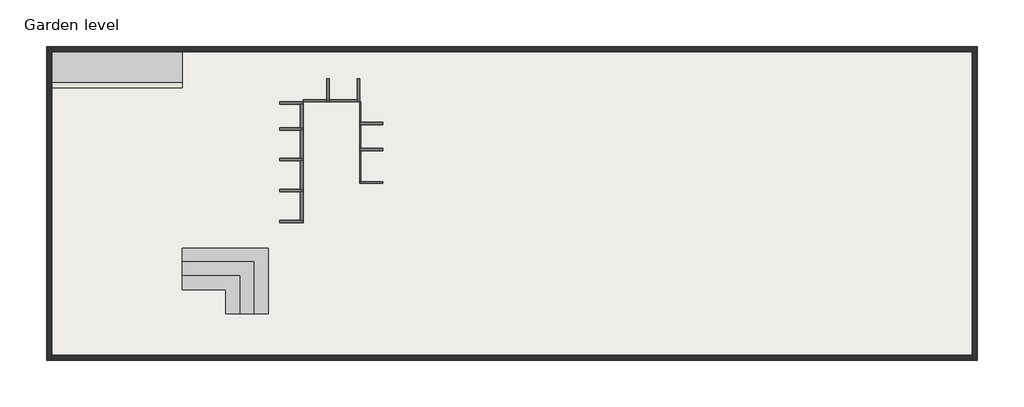
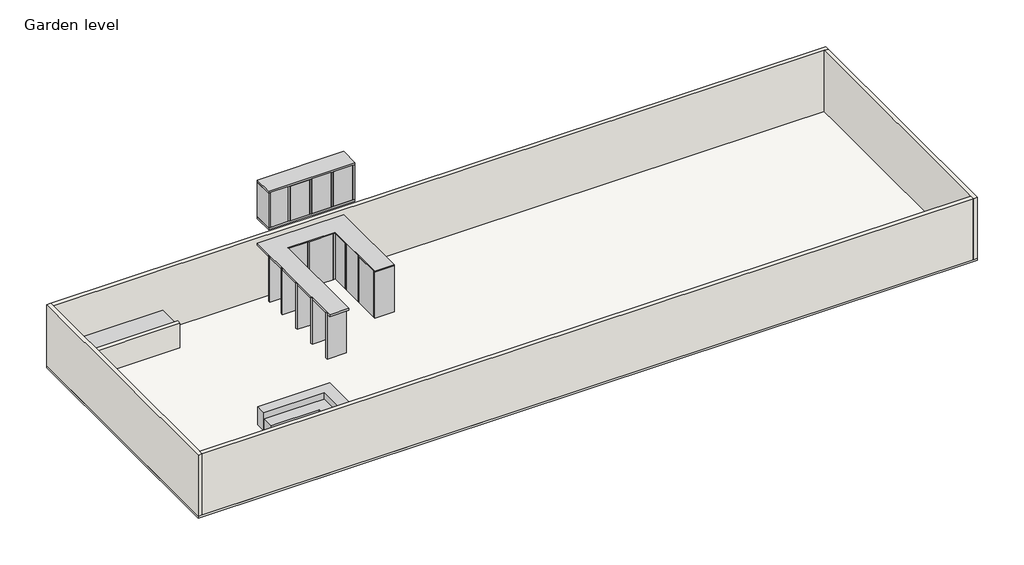
# One storey: 5 walls, 1 proxy, 1 slab.
"""IFC4 building model written with IfcOpenShell, lengths in millimetres."""

from ifc_helpers import new_model, si_unit, frame, origin, place, context, project, spatial, polyline, outline, extrude, faceted_brep, transform, mapped, element, save
from components import generic_models_1_generic_models_1_30c65cec

model = new_model("IFC4")

# Units and contexts
model_context = context("Model", 3, world=origin())
ifc_project = project(units=[si_unit("LENGTHUNIT", "METRE", prefix="MILLI")], contexts=[model_context])

# Site, building, storey
site = spatial("IfcSite", under=ifc_project)
building = spatial("IfcBuilding", under=site)
storey = spatial("IfcBuildingStorey", under=building, Name="Garden level", Elevation=-609.6)

# Proxy
placement = place(None, origin())
generic_models_1_generic_models_1_shape = generic_models_1_generic_models_1_30c65cec(model_context)
element("IfcBuildingElementProxy", 1, Name="Generic Models 1 : Generic Models 1", ObjectType="Generic Models 1 : Generic Models 1", at=placement, inside=storey, context=model_context, shape_type="MappedRepresentation", body=[
    mapped(generic_models_1_generic_models_1_shape, transform((0.0, 0.0, 0.0), x_axis=(1.0, 0.0, 0.0), y_axis=(0.0, 1.0, 0.0), z_axis=(0.0, 0.0, 1.0))),
])

# Slab
element("IfcSlab", 2, ObjectType="PARKING FLOOR", at=placement, inside=storey, context=model_context, shape_type="SweptSolid", body=[
    extrude(outline(polyline([(9314.7408773, 5508.9642852), (9314.7408773, -688.6357148), (-9074.8591227, -688.6357148), (-9074.8591227, 5508.9642852), (9314.7408773, 5508.9642852)])), frame((0.0, 0.0, -660.4), z_axis=(0.0, 0.0, 1.0), x_axis=(1.0, 0.0, 0.0)), (0.0, 0.0, 1.0), 50.8),
])

# Walls
element("IfcWall", 3, ObjectType="4\" WALL", at=placement, inside=storey, context=model_context, shape_type="Brep", body=[
    faceted_brep([(-8973.2591227, -688.6357148, -609.6), (-8973.2591227, -587.0357148, -609.6), (-8973.2591227, 4696.1642852, -609.6), (-8973.2591227, 4797.7642852, -609.6), (-8973.2591227, 5407.3642852, -609.6), (-8973.2591227, 5508.9642852, -609.6), (-8973.2591227, 5508.9642852, 914.4), (-8973.2591227, 5407.3642852, 914.4), (-8973.2591227, -587.0357148, 914.4), (-8973.2591227, -688.6357148, 914.4), (-9074.8591227, -688.6357148, -609.6), (-9074.8591227, -688.6357148, 914.4), (-9074.8591227, 5508.9642852, 914.4), (-9074.8591227, 5508.9642852, -609.6)], [[[0, 1, 2, 3, 4, 5, 6, 7, 8, 9]], [[10, 11, 12, 13]], [[5, 4, 3, 2, 1, 0, 10, 13]], [[9, 8, 7, 6, 12, 11]], [[6, 5, 13, 12]], [[0, 9, 11, 10]]]),
])
element("IfcWall", 4, ObjectType="4\" WALL", at=placement, inside=storey, context=model_context, shape_type="Brep", body=[
    faceted_brep([(-8973.2591227, 5407.3642852, -609.6), (9213.1408773, 5407.3642852, -609.6), (9314.7408773, 5407.3642852, -609.6), (9314.7408773, 5407.3642852, 914.4), (9213.1408773, 5407.3642852, 914.4), (-8973.2591227, 5407.3642852, 914.4), (-8973.2591227, 5508.9642852, -609.6), (-8973.2591227, 5508.9642852, 914.4), (9314.7408773, 5508.9642852, 914.4), (9314.7408773, 5508.9642852, -609.6)], [[[0, 1, 2, 3, 4, 5]], [[6, 7, 8, 9]], [[2, 1, 0, 6, 9]], [[5, 4, 3, 8, 7]], [[0, 5, 7, 6]], [[3, 2, 9, 8]]]),
])
element("IfcWall", 5, ObjectType="4\" WALL", at=placement, inside=storey, context=model_context, shape_type="Brep", body=[
    faceted_brep([(9213.1408773, 5407.3642852, -609.6), (9213.1408773, -587.0357148, -609.6), (9213.1408773, -688.6357148, -609.6), (9213.1408773, -688.6357148, 914.4), (9213.1408773, -587.0357148, 914.4), (9213.1408773, 5407.3642852, 914.4), (9314.7408773, 5407.3642852, -609.6), (9314.7408773, 5407.3642852, 914.4), (9314.7408773, -688.6357148, 914.4), (9314.7408773, -688.6357148, -609.6)], [[[0, 1, 2, 3, 4, 5]], [[6, 7, 8, 9]], [[2, 1, 0, 6, 9]], [[5, 4, 3, 8, 7]], [[0, 5, 7, 6]], [[3, 2, 9, 8]]]),
])
element("IfcWall", 6, ObjectType="4\" WALL", at=placement, inside=storey, context=model_context, shape_type="SweptSolid", body=[
    extrude(outline(polyline([(-8973.2591227, -587.0357148), (9213.1408773, -587.0357148), (9213.1408773, -688.6357148), (-8973.2591227, -688.6357148), (-8973.2591227, -587.0357148)])), frame((0.0, 0.0, -609.6), z_axis=(0.0, 0.0, 1.0), x_axis=(1.0, 0.0, 0.0)), (0.0, 0.0, 1.0), 1524.0),
])
element("IfcWall", 7, ObjectType="4\" WALL", at=placement, inside=storey, context=model_context, shape_type="SweptSolid", body=[
    extrude(outline(polyline([(-6395.1591227, 4696.1642852), (-8973.2591227, 4696.1642852), (-8973.2591227, 4797.7642852), (-6395.1591227, 4797.7642852), (-6395.1591227, 4696.1642852)])), frame((0.0, 0.0, -609.6), z_axis=(0.0, 0.0, 1.0), x_axis=(1.0, 0.0, 0.0)), (0.0, 0.0, 1.0), 609.6),
])

save(model, "model.ifc")

# Revit data of these elements
# Grids (mm)
#   "1": line (8755.941, 7644.224) -> (8755.941, -2355.226)
#   "2": line (5542.841, -2355.226) -> (5542.841, 7644.224)
#   "3": line (2342.441, -2355.226) -> (2342.441, 7644.224)
#   "4": line (-2280.359, -2355.226) -> (-2280.359, 7644.224)
#   "5": line (-4579.059, -2355.226) -> (-4579.059, 7644.224)
#   "A": line (-11144.212, 4988.264) -> (11854.741, 4988.264)
#   "B": line (-11144.212, 276.564) -> (11702.341, 276.564)
# Type "PARKING FLOOR"
#   Assembly Code = "B1010"
#   Function = 0
#   Layers, outside or top first: 0' - 2" "PARKING FLOOR" (function 1)
# Type "4\" WALL"
#   Assembly Code = "B2010"
#   Layers, outside or top first: 0' - 4" "Brick, Common" (function 1)
# Element 1 (IfcBuildingElementProxy, "Generic Models 1 : Generic Models 1")
#   Phase Created = New Construction
#   Materials on its faces: "Grass"
# Element 2 (IfcSlab, "PARKING FLOOR")
#   Height Offset From Level = 0' - 0"
#   Phase Created = New Construction
#   Materials on its faces: "PARKING FLOOR"
# Elements 3, 4, 5, 6 (IfcWall, "4\" WALL")
#   Top Offset = 0' - 0"
#   Base Offset = 0' - 0"
#   Unconnected Height = 5' - 0"
#   wall height = 5' - 0"
#   Phase Created = New Construction
#   Base Constraint = Garden level
#   Materials on its faces: "Brick, Common"
# Element 7 (IfcWall, "4\" WALL")
#   Top Offset = 0' - 0"
#   Base Offset = 0' - 0"
#   Unconnected Height = 2' - 0"
#   wall height = 2' - 0"
#   Phase Created = New Construction
#   Base Constraint = Garden level
#   Materials on its faces: "Brick, Common"
# Materials
#   "PARKING FLOOR": class "Generic", colour RGB 173 180 185, transparency 0, Cost = 0
#   "Brick, Common": class "Masonry", colour RGB 170 98 104, transparency 0, Description = "Common brick", Cost = 0
#   "Grass": class "Generic", colour RGB 27 35 14, transparency 0, Description = "Physical material.", Cost = 0
